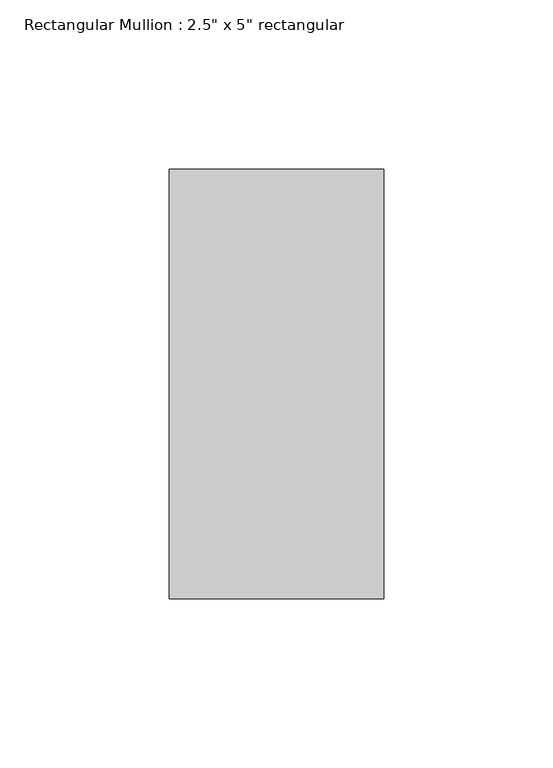
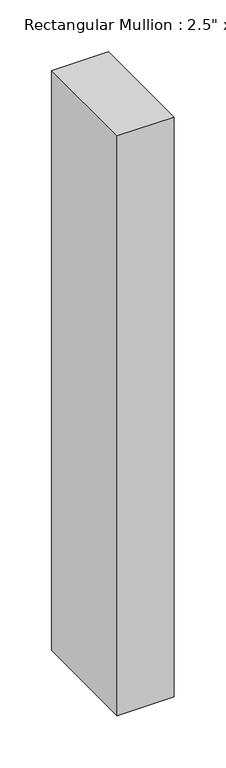
"""IFC4 building model written with IfcOpenShell, lengths in millimetres: member geometry."""

from ifc_helpers import new_model, si_unit, frame, origin, place, context, project, spatial, polyline, outline, extrude, source, transform, mapped, element, save


def member_ee3d4f96(model_context):
    return source(origin(), model_context, "Body", "SweptSolid", [
        extrude(outline(polyline([(0.0, 63.5), (0.0, -63.5), (-63.5, -63.5), (-63.5, 63.5), (0.0, 63.5)])), frame((0.0, 0.0, -684.8022733), z_axis=(0.0, 0.0, 1.0), x_axis=(1.0, 0.0, 0.0)), (0.0, 0.0, 1.0), 684.8022733),
    ])


if __name__ == "__main__":
    model = new_model("IFC4")
    model_context = context("Model", 3, world=origin())
    ifc_project = project(units=[si_unit("LENGTHUNIT", "METRE", prefix="MILLI")], contexts=[model_context])
    site = spatial("IfcSite", under=ifc_project)
    building = spatial("IfcBuilding", under=site)
    placement = place(None, origin())
    member_shape = member_ee3d4f96(model_context)
    element("IfcMember", 1, ObjectType="Rectangular Mullion : 2.5\" x 5\" rectangular", at=placement, inside=building, context=model_context, shape_type="MappedRepresentation", body=[
        mapped(member_shape, transform((0.0, 0.0, 0.0), x_axis=(1.0, 0.0, 0.0), y_axis=(0.0, 1.0, 0.0), z_axis=(0.0, 0.0, 1.0))),
    ])
    save(model, "model.ifc")

# Revit data of these elements
# Type "Rectangular Mullion : 2.5\" x 5\" rectangular"
#   built-in parameter 1007304 = 0.416667 (stored number, unit not read)
#   built-in parameter 1007301 = 0.104167 (stored number, unit not read)
#   built-in parameter 1007300 = 0.104167 (stored number, unit not read)
# Element 1 (IfcMember, "Rectangular Mullion : 2.5\" x 5\" rectangular")
#   Materials on its faces: "Aluminum"
# Materials
#   "Aluminum": class "Metal", colour RGB 247 247 247, transparency 0, Description = "Aluminum 6061", Cost = 0
